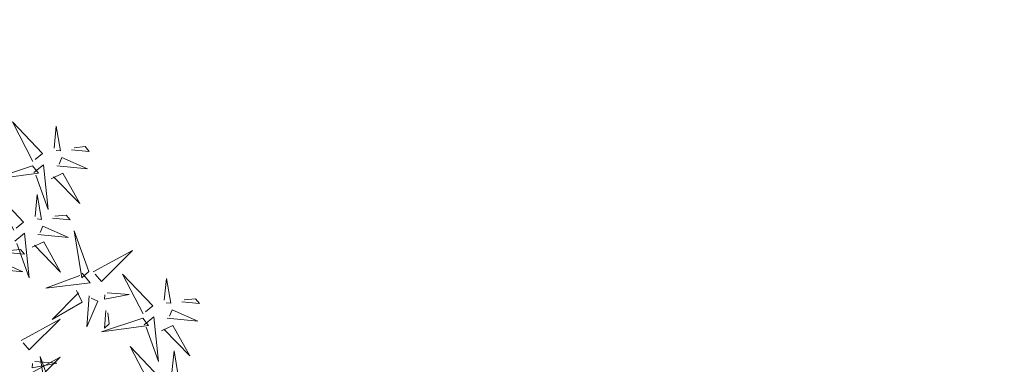
# Model space of a CAD drawing. Units: inches. Extents: x 1704 to 6393, y -157 to 1172.
# Tile 72 of 122: x 1920 to 1954, y 1033 to 1045. Entities that reach past the tile are written whole.
import ezdxf

# ---------------------------------------------------------------- set-up
doc = ezdxf.new("R2010")
doc.units = ezdxf.units.IN
doc.header["$MEASUREMENT"] = 0
for name, color, linetype, lineweight in [('A-ANNO-DIMS', 7, 'Continuous', 13), ('L-shrub', 74, 'Continuous', 18), ('L-tree', 102, 'Continuous', 18)]:
    doc.layers.add(name, color=color, linetype=linetype, lineweight=lineweight)
doc.styles.get("Standard").update_dxf_attribs({"font": 'arial.ttf'})
doc.dimstyles.get("Standard").update_dxf_attribs({"dimtxt": 6, "dimasz": 2, "dimexe": 0.18, "dimexo": 0.0625, "dimgap": 0.09, "dimtad": 0, "dimtih": 1, "dimtoh": 1, "dimdec": 1, "dimzin": 0, "dimdsep": 46, "dimlunit": 3, "dimtxsty": 'Standard', "dimblk": 'ARCHTICK', "dimcen": 0.09, "dimadec": 0, "dimazin": 0, "dimtfac": 1, "dimtdec": 1, "dimtofl": 0, "dimtmove": 0, "dimatfit": 3, "dimfxl": 1, "dimtolj": 1, "dimtzin": 0, "dimarcsym": 0})

# ---------------------------------------------------------------- blocks, each defined once
blk = doc.blocks.new('bamboo')
at = {"layer": 'L-shrub'}
for points in [[(813.3, -626.1), (802.7, -736.2), (843.2, -644.9), (820.4, -634.7)], [(952.3, -704), (1094.2, -630.5), (980.7, -738.5), (959.4, -712.7)], [(1182.3, -770.7), (1132.9, -623.1), (1156.5, -792), (1182.3, -770.7)], [(871.6, -679.4), (865.6, -742.3), (882.9, -728.1), (878.8, -688)], [(1198, -772.2), (1339.9, -698.7), (1226.5, -806.7), (1205.1, -780.8)], [(419.5, -729.9), (495.9, -870.2), (385.6, -759), (411, -737.1)], [(556, -729.9), (632.4, -870.2), (522.1, -759), (547.5, -737.1)], [(912.2, -708.1), (940.6, -742.6), (780.4, -758.8), (903.6, -715.2)], [(480.9, -779.7), (474.9, -858.4), (457.9, -770), (473.7, -771.2)], [(890.5, -769.5), (910.3, -811.1), (801.3, -871.9), (897.6, -778.1)], [(1158, -776.3), (1186.4, -810.8), (1026.2, -827), (1149.3, -783.4)], [(352.4, -850.5), (499, -798.1), (330.6, -825.1), (352.4, -850.5)], [(936.1, -789.8), (925.6, -899.8), (966.1, -808.5), (943.2, -798.4)], [(1000.5, -780.1), (1079.1, -787.7), (990.4, -802.9), (991.9, -787.2)], [(735.1, -928.5), (693.9, -949.2), (630.8, -841.5), (726.6, -935.8)], [(796.9, -949), (763, -978.1), (743.5, -818.2), (789.6, -940.5)], [(994.5, -843), (988.5, -905.9), (1005.7, -891.7), (1001.6, -851.6)], [(1136.2, -837.6), (1156, -879.2), (1047.1, -940.1), (1143.3, -846.3)], [(1181.9, -857.9), (1171.4, -968), (1211.8, -876.7), (1189, -866.6)], [(1246.3, -848.3), (1324.9, -855.9), (1236.2, -871.1), (1237.7, -855.4)], [(1240.3, -911.2), (1234.3, -974.1), (1251.5, -959.9), (1247.4, -919.8)], [(803, -973.2), (949.5, -920.8), (781.1, -947.8), (803, -973.2)], [(715.7, -974.6), (605.5, -966.3), (697.6, -1004.9), (707.3, -981.8)], [(636.2, -1166.1), (586.8, -1018.5), (610.3, -1187.4), (636.2, -1166.1)], [(801.8, -988.9), (878.2, -1129.3), (767.9, -1018.1), (793.3, -996.2)], [(663.7, -1034), (600.7, -1029.3), (615.2, -1046.2), (655.2, -1041.3)], [(726.7, -1038.7), (720.7, -1117.5), (703.7, -1029.1), (719.4, -1030.3)], [(651.9, -1167.6), (793.8, -1094.1), (680.3, -1202.1), (659, -1176.3)], [(392.5, -1194.9), (534.4, -1121.4), (420.9, -1229.4), (399.6, -1203.5)], [(611.8, -1171.7), (640.3, -1206.2), (480.1, -1222.4), (603.2, -1178.8)], [(590.1, -1233.1), (609.9, -1274.7), (501, -1335.5), (597.2, -1241.7)], [(440.8, -1271), (519.4, -1278.6), (430.7, -1293.8), (432.2, -1278.1)], [(635.8, -1253.4), (625.3, -1363.4), (665.7, -1272.1), (642.9, -1262)], [(700.2, -1243.7), (778.8, -1251.3), (690.1, -1266.6), (691.6, -1250.8)], [(694.2, -1306.6), (688.2, -1369.5), (705.4, -1355.3), (701.3, -1315.3)]]:
    blk.add_lwpolyline(points, dxfattribs=at)
blk = doc.blocks.new('_ArchTick')
at = {"color": 0, "linetype": 'ByBlock', "const_width": 0.15}
blk.add_lwpolyline([(-0.5, -0.5), (0.5, 0.5)], dxfattribs=at)
blk = doc.blocks.new('*D80')
at = {"layer": 'A-ANNO-DIMS', "color": 0, "lineweight": -2, "transparency": 16777216}
for p, q in [((2018.966, 1025.001), (2018.966, 1029.096)), ((2045.487, 1025.001), (2045.487, 1029.096)), ((2018.966, 1028.916), (2016.966, 1028.916)), ((2045.487, 1028.916), (2018.966, 1028.916))]:
    blk.add_line(p, q, dxfattribs=at)
at = {"layer": 'Defpoints', "color": 0, "lineweight": -3, "transparency": 16777216}
for p in [(2018.966, 1028.916), (2018.966, 1024.938), (2045.487, 1024.938)]:
    blk.add_point(p, dxfattribs=at)
at = {"layer": 'A-ANNO-DIMS', "color": 0, "lineweight": -2, "transparency": 16777216, "xscale": 2, "yscale": 2, "zscale": 2, "rotation": 180}
blk.add_blockref('_ArchTick', (2018.966, 1028.916), dxfattribs=at)
at = {"layer": 'A-ANNO-DIMS', "color": 0, "lineweight": -2, "transparency": 16777216, "xscale": 2, "yscale": 2, "zscale": 2}
blk.add_blockref('_ArchTick', (2045.487, 1028.916), dxfattribs=at)
at = {"layer": 'A-ANNO-DIMS', "color": 0, "transparency": 16777216, "insert": (1967.173, 1028.916), "char_height": 6, "attachment_point": 5}
blk.add_mtext('\\A1;AUTUMN SHRUB 27 TYP.', dxfattribs=at)
blk = doc.blocks.new('*D94')
at = {"layer": 'A-ANNO-DIMS', "color": 0, "lineweight": -2, "transparency": 16777216}
for p, q in [((1898.349, 895.275), (1898.349, 1105.287)), ((2073.349, 895.275), (2073.349, 1105.287)), ((1898.349, 1105.107), (1979.39, 1105.107)), ((2073.349, 1105.107), (1992.307, 1105.107))]:
    blk.add_line(p, q, dxfattribs=at)
at = {"layer": 'Defpoints', "color": 0, "lineweight": -3, "transparency": 16777216}
for p in [(2073.349, 1105.107), (1898.349, 895.213), (2073.349, 895.213)]:
    blk.add_point(p, dxfattribs=at)
at = {"layer": 'A-ANNO-DIMS', "color": 0, "lineweight": -2, "transparency": 16777216, "xscale": 2, "yscale": 2, "zscale": 2, "rotation": 180}
blk.add_blockref('_ArchTick', (1898.349, 1105.107), dxfattribs=at)
at = {"layer": 'A-ANNO-DIMS', "color": 0, "lineweight": -2, "transparency": 16777216, "xscale": 2, "yscale": 2, "zscale": 2}
blk.add_blockref('_ArchTick', (2073.349, 1105.107), dxfattribs=at)
at = {"layer": 'A-ANNO-DIMS', "color": 0, "transparency": 16777216, "insert": (1985.849, 1105.107), "char_height": 6, "attachment_point": 5}
blk.add_mtext('\\A1;175', dxfattribs=at)

msp = doc.modelspace()

# ---------------------------------------------------------------- block references
at = {"layer": 'L-tree', "xscale": 0.0095734028514679, "yscale": 0.0095734028514679, "zscale": 0.0095734028514679, "rotation": 89.99999999999996}
msp.add_blockref('bamboo', (1913.269, 1028.796), dxfattribs=at)

# ---------------------------------------------------------------- dimensions: what is measured, and where the dimension line sits
at = {"layer": 'A-ANNO-DIMS'}
dim = msp.add_linear_dim(base=(2073.349, 1105.107), p1=(1898.349, 895.213), p2=(2073.349, 895.213), dimstyle='Standard', override={"dimdec": 0, "dimlfac": 1, "dimrnd": 0, "dimzin": 0, "dimdsep": 46, "dimlunit": 2}, dxfattribs=at)
dim.commit()
dim.dimension.update_dxf_attribs({"geometry": '*D94', "text_midpoint": (1985.849, 1105.107)})
dim = msp.add_linear_dim(base=(2018.966, 1028.916), p1=(2045.487, 1024.938), p2=(2018.966, 1024.938), angle=180, text='AUTUMN SHRUB <> TYP.', dimstyle='Standard', override={"dimdec": 0, "dimlfac": 1, "dimrnd": 0, "dimzin": 0, "dimdsep": 46, "dimlunit": 2}, dxfattribs=at)
dim.commit()
dim.dimension.update_dxf_attribs({"geometry": '*D80', "text_midpoint": (1967.173, 1028.916)})

doc.saveas('drawing.dxf')
